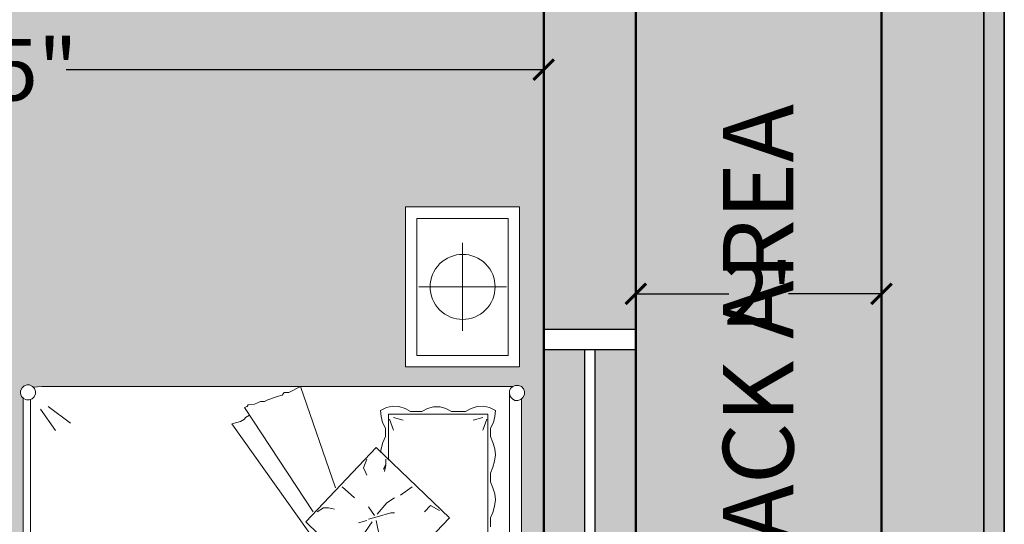
# Model space of a CAD drawing. Units: inches. Extents: x 528 to 2620, y -1066 to 798.
# Tile 15 of 41: x 848 to 944, y 623 to 672. Entities that reach past the tile are written whole.
import ezdxf

# ---------------------------------------------------------------- set-up
doc = ezdxf.new("R2010")
doc.units = ezdxf.units.IN
doc.header["$MEASUREMENT"] = 0
for name, color, linetype, lineweight in [('A-ANNO-DIMS', 2, 'Continuous', 18), ('A-AREA-IDEN', 7, 'Continuous', 18), ('A-FURN', 30, 'Continuous', 18), ('A-GLAZ', 3, 'Continuous', 25), ('A-WALL', 7, 'Continuous', 50), ('A-WALL-PATT', 8, 'Continuous', 13), ('C-PROP', 5, 'Continuous', 35)]:
    doc.layers.add(name, color=color, linetype=linetype, lineweight=lineweight)
doc.styles.get("Standard").update_dxf_attribs({"font": 'arial.ttf'})
doc.dimstyles.get("Standard").update_dxf_attribs({"dimtxt": 6, "dimasz": 2, "dimexe": 0.18, "dimexo": 0.0625, "dimgap": 0.09, "dimtad": 0, "dimtih": 1, "dimtoh": 1, "dimdec": 1, "dimzin": 0, "dimdsep": 46, "dimlunit": 3, "dimtxsty": 'Standard', "dimblk": 'ARCHTICK', "dimcen": 0.09, "dimadec": 0, "dimazin": 0, "dimtfac": 1, "dimtdec": 1, "dimtofl": 0, "dimtmove": 0, "dimatfit": 3, "dimfxl": 1, "dimtolj": 1, "dimtzin": 0, "dimarcsym": 0})

# ---------------------------------------------------------------- blocks, each defined once
blk = doc.blocks.new('d-bed-3')
at = {"color": 0, "linetype": 'ByBlock'}
for p, q in [((0, 0), (0, -0.5)), ((0.7, 0), (0, 0)), ((0.7, -0.5), (0.7, 0)), ((0.7817, -0.0054), (0.7857, 0.0078)), ((0.7817, -0.0054), (0.7857, 0.0078)), ((0.7857, 0.0078), (0.7968, 0.0166)), ((0.7857, 0.0078), (0.7968, 0.0166)), ((0.7968, 0.0166), (0.8078, 0.0211)), ((0.7968, 0.0166), (0.8078, 0.0211)), ((0.8078, 0.0211), (0.8209, 0.0211)), ((0.8078, 0.0211), (0.8209, 0.0211)), ((0.8209, 0.0211), (0.8349, 0.0144)), ((0.8209, 0.0211), (0.8349, 0.0144)), ((0.8349, 0.0144), (0.8409, 0.0078)), ((0.8349, 0.0144), (0.8429, 0.0056)), ((0.8389, 0.0078), (2.7305, 0.0078)), ((0.8409, 0.0078), (2.7305, 0.0078)), ((0.8429, 0.0056), (0.848, -0.0077)), ((0.7817, -0.0187), (0.7817, -0.0054)), ((0.7817, -0.0187), (0.7817, -0.0054)), ((0.7857, -0.0297), (0.7817, -0.0187)), ((0.7857, -0.0297), (0.7817, -0.0187)), ((0.7857, -2.0939), (0.7857, -0.0297)), ((0.7948, -0.0408), (0.7857, -0.0297)), ((0.7857, -0.032), (0.7857, -2.0939)), ((0.8058, -0.0452), (0.7948, -0.0408)), ((0.8319, -0.0408), (0.8188, -0.0452)), ((0.8409, -0.032), (0.8319, -0.0408)), ((0.848, -0.0209), (0.8409, -0.032)), ((0.848, -0.0077), (0.848, -0.0209)), ((0.05, -0.05), (0.05, -0.45)), ((0.65, -0.05), (0.05, -0.05)), ((0.35, -0.0576), (0.35, -0.4424)), ((0.65, -0.45), (0.65, -0.05)), ((0.8188, -0.0452), (0.8058, -0.0452)), ((2.7525, -0.0452), (0.8188, -0.0452)), ((0.8781, -0.1325), (0.8911, -0.1059)), ((0.8911, -0.1059), (0.9182, -0.1082)), ((0.9182, -0.1082), (0.9443, -0.1148)), ((0.9443, -0.1148), (0.9684, -0.128)), ((0.9684, -0.128), (1.0056, -0.128)), ((1.0056, -0.128), (1.0317, -0.117)), ((1.0317, -0.117), (1.0588, -0.1082)), ((1.0588, -0.1082), (1.0849, -0.1059)), ((1.0849, -0.1059), (1.113, -0.1104)), ((1.113, -0.1104), (1.1401, -0.117)), ((1.1401, -0.117), (1.1662, -0.128)), ((1.1662, -0.128), (1.2034, -0.128)), ((1.2034, -0.128), (1.2295, -0.117)), ((1.2295, -0.117), (1.2566, -0.1082)), ((1.2566, -0.1082), (1.2827, -0.1059)), ((1.2827, -0.1059), (1.3108, -0.1104)), ((1.3108, -0.1104), (1.3379, -0.117)), ((1.3379, -0.117), (1.362, -0.128)), ((1.362, -0.128), (1.4012, -0.128)), ((0.8721, -0.159), (0.8781, -0.1325)), ((0.8741, -0.1866), (0.8721, -0.159)), ((0.9072, -0.5753), (0.9072, -0.1391)), ((0.9072, -0.1391), (1.6763, -0.1391)), ((0.9223, -0.1612), (0.9333, -0.2042)), ((0.9293, -0.1435), (0.9775, -0.1612)), ((0.8831, -0.2131), (0.8741, -0.1866)), ((0.8962, -0.2374), (0.8831, -0.2131)), ((0.1576, -0.25), (0.5424, -0.25)), ((0.8962, -0.2992), (0.8962, -0.2374)), ((0.8831, -0.3235), (0.8962, -0.2992)), ((0.8761, -0.3489), (0.8831, -0.3235)), ((1.0538, -0.6294), (1.362, -0.3081)), ((1.362, -0.3081), (1.619, -0.5532)), ((0.8761, -0.3776), (0.8761, -0.3489)), ((0.8831, -0.4041), (0.8761, -0.3776)), ((1.3289, -0.3511), (1.3068, -0.3909)), ((0.8962, -0.4284), (0.8831, -0.4041)), ((0.8962, -0.4781), (0.8962, -0.4284)), ((1.3068, -0.3909), (1.3349, -0.4174)), ((0.05, -0.45), (0.65, -0.45)), ((1.2255, -0.4715), (1.2626, -0.5223)), ((0, -0.5), (0.7, -0.5)), ((0.8741, -0.5289), (0.8831, -0.5024)), ((0.8831, -0.5024), (0.8962, -0.4781)), ((0.9223, -0.5532), (0.9333, -0.5113)), ((0.8721, -0.5576), (0.8741, -0.5289)), ((0.8781, -0.5841), (0.8721, -0.5576)), ((0.9293, -0.5709), (0.9775, -0.5532)), ((1.2957, -0.5819), (1.2737, -0.5488)), ((1.3399, -0.5643), (1.3399, -0.5488)), ((0.8911, -0.6096), (0.8781, -0.5841)), ((1.109, -0.5753), (0.9072, -0.5753)), ((0.9443, -0.6007), (0.9182, -0.6073)), ((0.9684, -0.5886), (0.9443, -0.6007)), ((1.0056, -0.5886), (0.9684, -0.5886)), ((1.0317, -0.5996), (1.0056, -0.5886)), ((1.0588, -0.6073), (1.0317, -0.5996)), ((1.105, -0.5864), (1.1271, -0.5864)), ((1.1271, -0.5864), (1.1482, -0.5974)), ((1.1482, -0.5974), (1.1311, -0.5864)), ((1.1311, -0.5864), (1.1592, -0.593)), ((1.3459, -0.625), (1.2957, -0.5819)), ((1.357, -0.625), (1.3399, -0.5643)), ((0.9182, -0.6073), (0.8911, -0.6096)), ((1.3791, -0.9365), (1.0538, -0.6294)), ((1.0759, -0.6096), (1.0588, -0.6073)), ((1.3138, -0.6626), (1.351, -0.6361)), ((1.368, -0.6626), (1.357, -0.625)), ((1.3731, -0.6294), (1.4453, -0.614)), ((1.3791, -0.6471), (1.4453, -0.6913)), ((1.105, -0.6692), (1.1421, -0.6846)), ((1.1421, -0.6846), (1.1642, -0.6736)), ((1.1642, -0.6736), (1.1753, -0.6692)), ((1.3731, -0.6692), (1.3841, -0.7067)), ((1.2255, -0.7785), (1.2737, -0.7244)), ((1.3791, -0.9365), (1.5357, -0.7763)), ((0.7857, -0.9607), (1.2295, -0.8072)), ((0.9504, -1.2611), (1.5708, -0.8183)), ((1.3178, -0.8382), (1.3239, -0.8117)), ((1.3178, -0.8602), (1.3178, -0.8382)), ((1.3349, -0.8879), (1.3178, -0.8602)), ((0.8781, -1.2059), (1.3349, -0.9055)), ((0.8128, -1.0115), (0.7857, -0.9607)), ((0.8128, -1.0325), (0.8128, -1.0115)), ((0.8239, -1.0414), (0.8128, -1.0325)), ((0.8299, -1.0635), (0.8239, -1.0414)), ((0.8349, -1.0745), (0.8299, -1.0635)), ((0.845, -1.1032), (0.8349, -1.0745)), ((0.852, -1.1187), (0.845, -1.1032)), ((0.852, -1.1363), (0.852, -1.1187)), ((0.863, -1.1617), (0.852, -1.1363)), ((0.867, -1.1905), (0.863, -1.1617)), ((0.8741, -1.1949), (0.867, -1.1905)), ((0.8781, -1.2059), (0.8741, -1.1949)), ((0.9223, -1.2015), (0.9112, -1.1838)), ((0.9293, -1.2059), (0.9223, -1.2015)), ((0.9403, -1.2236), (0.9293, -1.2059)), ((0.9443, -1.2391), (0.9403, -1.2236)), ((0.9504, -1.2611), (0.9443, -1.2391)), ((0.8741, -2.0673), (0.9464, -1.9691)), ((0.8851, -2.1005), (0.9795, -2.0342)), ((0.7888, -2.1317), (0.7857, -2.0939)), ((0.7857, -2.0939), (0.7887, -2.1303)), ((0.7797, -2.148), (0.7857, -2.1347)), ((0.7797, -2.148), (0.7857, -2.1347)), ((0.7797, -2.159), (0.7797, -2.148)), ((0.7797, -2.148), (0.7797, -2.159)), ((0.7857, -2.1347), (0.7948, -2.1259)), ((0.7857, -2.1347), (0.7888, -2.1317)), ((0.7948, -2.1259), (0.8078, -2.1215)), ((0.8078, -2.1215), (0.8188, -2.1215)), ((0.8188, -2.1215), (0.8319, -2.1281)), ((0.8319, -2.1281), (0.8409, -2.1369)), ((0.8409, -2.1369), (0.845, -2.1502)), ((2.7264, -2.1436), (0.845, -2.1436)), ((0.845, -2.1502), (0.845, -2.1612)), ((0.7837, -2.1723), (0.7797, -2.159)), ((0.7837, -2.1723), (0.7797, -2.159)), ((0.7927, -2.1811), (0.7837, -2.1723)), ((0.7927, -2.1811), (0.7837, -2.1723)), ((0.8058, -2.1877), (0.7927, -2.1811)), ((0.8058, -2.1877), (0.7927, -2.1811)), ((0.8168, -2.1877), (0.8058, -2.1877)), ((0.8168, -2.1877), (0.8058, -2.1877)), ((0.8299, -2.1833), (0.8168, -2.1877)), ((0.8299, -2.1833), (0.8168, -2.1877)), ((0.8389, -2.1745), (0.8299, -2.1833)), ((0.8367, -2.1767), (0.8299, -2.1833)), ((2.7327, -2.1767), (0.8367, -2.1767)), ((0.845, -2.1612), (0.8389, -2.1745)), ((0.8389, -2.1767), (2.7305, -2.1767))]:
    blk.add_line(p, q, dxfattribs=at)
blk.add_ellipse((0.35, -0.25), major_axis=(-0.1007, 0.1007), ratio=1, dxfattribs=at)
blk = doc.blocks.new('_ArchTick')
at = {"color": 0, "linetype": 'ByBlock', "const_width": 0.15}
blk.add_lwpolyline([(-0.5, -0.5), (0.5, 0.5)], dxfattribs=at)
blk = doc.blocks.new('*D27')
at = {"layer": 'A-ANNO-DIMS', "color": 0, "lineweight": -2, "transparency": 16777216}
for p, q in [((778.559, 667.76), (778.559, 666.811)), ((899.059, 667.76), (899.059, 666.811)), ((778.559, 666.991), (825.201, 666.991)), ((899.059, 666.991), (852.418, 666.991))]:
    blk.add_line(p, q, dxfattribs=at)
at = {"layer": 'Defpoints', "color": 0, "transparency": 16777216}
for p in [(778.559, 667.823), (899.059, 667.823), (899.059, 666.991)]:
    blk.add_point(p, dxfattribs=at)
at = {"layer": 'A-ANNO-DIMS', "color": 0, "lineweight": -2, "transparency": 16777216, "xscale": 2, "yscale": 2, "zscale": 2, "rotation": 180}
blk.add_blockref('_ArchTick', (778.559, 666.991), dxfattribs=at)
at = {"layer": 'A-ANNO-DIMS', "color": 0, "lineweight": -2, "transparency": 16777216, "xscale": 2, "yscale": 2, "zscale": 2}
blk.add_blockref('_ArchTick', (899.059, 666.991), dxfattribs=at)
at = {"layer": 'A-ANNO-DIMS', "color": 0, "transparency": 16777216, "insert": (838.809, 666.991), "char_height": 6, "attachment_point": 5}
blk.add_mtext('\\A1;10\'-0.5"', dxfattribs=at)
blk = doc.blocks.new('*D39')
at = {"layer": 'A-ANNO-DIMS', "color": 0, "lineweight": -2, "transparency": 16777216}
for p, q in [((908.059, 645.184), (908.059, 645.301)), ((908.059, 645.121), (917.158, 645.121)), ((932.059, 645.121), (922.961, 645.121)), ((932.059, 645.184), (932.059, 645.301))]:
    blk.add_line(p, q, dxfattribs=at)
at = {"layer": 'Defpoints', "color": 0, "transparency": 16777216}
for p in [(908.059, 645.121), (932.059, 645.121), (932.059, 645.121)]:
    blk.add_point(p, dxfattribs=at)
at = {"layer": 'A-ANNO-DIMS', "color": 0, "lineweight": -2, "transparency": 16777216, "xscale": 2, "yscale": 2, "zscale": 2, "rotation": 180}
blk.add_blockref('_ArchTick', (908.059, 645.121), dxfattribs=at)
at = {"layer": 'A-ANNO-DIMS', "color": 0, "lineweight": -2, "transparency": 16777216, "xscale": 2, "yscale": 2, "zscale": 2}
blk.add_blockref('_ArchTick', (932.059, 645.121), dxfattribs=at)
at = {"layer": 'A-ANNO-DIMS', "color": 0, "transparency": 16777216, "insert": (920.059, 645.121), "char_height": 6, "attachment_point": 5}
blk.add_mtext("\\A1;2'", dxfattribs=at)
blk = doc.blocks.new('WIN-1200')
for p, q in [((677.559, 718.922), (725.559, 718.922)), ((677.559, 709.922), (677.559, 718.922)), ((679.559, 709.922), (679.559, 718.922)), ((723.559, 718.922), (723.559, 709.922)), ((725.559, 718.922), (725.559, 709.922)), ((679.559, 714.922), (723.559, 714.922)), ((679.559, 713.922), (723.559, 713.922)), ((725.559, 709.922), (677.559, 709.922))]:
    blk.add_line(p, q)

msp = doc.modelspace()

# ---------------------------------------------------------------- hatches: boundary and pattern name
at = {"layer": 'A-WALL-PATT', "transparency": 33554687}
h = msp.add_hatch(color=256, dxfattribs=at)
h.dxf.hatch_style = 1
h.paths.add_polyline_path([(944.059, 753.922), (584.059, 753.922), (584.059, 208.922), (608.059, 208.922), (608.059, 210.922), (586.059, 210.922), (586.059, 751.922), (942.059, 751.922), (942.059, 210.922), (728.059, 210.922), (728.059, 208.922), (944.059, 208.922)])
h = msp.add_hatch(color=256, dxfattribs=at)
h.dxf.hatch_style = 1
h.paths.add_polyline_path([(942.059, 751.922), (586.059, 751.922), (586.059, 210.922), (608.059, 210.922), (608.059, 220.922), (596.059, 220.922), (596.059, 741.922), (932.059, 741.922), (932.059, 220.922), (770.059, 220.922), (728.059, 220.922), (728.059, 210.922), (942.059, 210.922)])
at = {"layer": 'A-WALL-PATT', "transparency": 33554475}
h = msp.add_hatch(color=256, dxfattribs=at)
h.dxf.hatch_style = 1
h.paths.add_polyline_path([(620.059, 718.922), (908.059, 718.922), (908.059, 268.922), (770.059, 268.922), (770.059, 220.922), (932.059, 220.922), (932.059, 741.922), (596.059, 741.922), (596.059, 391.422), (620.059, 391.422)])
at = {"layer": 'A-WALL-PATT', "transparency": 33554687}
h = msp.add_hatch(color=256, dxfattribs=at)
h.dxf.hatch_style = 1
h.paths.add_polyline_path([(861.059, 273.922), (817.059, 273.922), (817.059, 272.922), (861.059, 272.922)])
h.paths.add_polyline_path([(817.059, 277.922), (815.059, 277.922), (815.059, 268.922), (817.059, 268.922)])
h.paths.add_polyline_path([(908.059, 397.922), (899.059, 397.922), (899.059, 395.922), (908.059, 395.922)])
h.paths.add_polyline_path([(908.059, 443.922), (899.059, 443.922), (899.059, 441.922), (908.059, 441.922)])
h.paths.add_polyline_path([(904.059, 441.922), (903.059, 441.922), (903.059, 397.922), (904.059, 397.922)])
h.paths.add_polyline_path([(625.059, 561.422), (624.059, 561.422), (624.059, 537.422), (625.059, 537.422)])
h.paths.add_polyline_path([(648.747, 334.444), (720.045, 334.444), (720.045, 344.998), (648.747, 344.998)], flags=9)
h.paths.add_polyline_path([(819.733, 323.153), (880.328, 323.153), (880.328, 333.708), (819.733, 333.708)], flags=9)
h.paths.add_polyline_path([(779.898, 680.607), (821.764, 680.607), (821.764, 691.169), (779.898, 691.169)], flags=9)
h.paths.add_polyline_path([(779.876, 692.362), (817.138, 692.362), (817.138, 703.058), (779.876, 703.058)], flags=9)
h.paths.add_polyline_path([(799.994, 453.884), (860.589, 453.884), (860.589, 464.439), (799.994, 464.439)], flags=9)
h.paths.add_polyline_path([(650.866, 539.397), (708.781, 539.397), (708.781, 549.952), (650.866, 549.952)], flags=9)
h.paths.add_polyline_path([(788.504, 612.01), (849.099, 612.01), (849.099, 622.565), (788.504, 622.565)], flags=9)
h.paths.add_polyline_path([(639.539, 648.31), (700.134, 648.31), (700.134, 658.865), (639.539, 658.865)], flags=9)
h.paths.add_polyline_path([(648.913, 346.09), (747.706, 346.09), (747.706, 356.778), (648.913, 356.778)], flags=9)
h.paths.add_polyline_path([(676.857, 450.66), (746.735, 450.66), (746.735, 461.355), (676.857, 461.355)], flags=9)
h.paths.add_polyline_path([(819.711, 334.947), (865.526, 334.947), (865.526, 345.636), (819.711, 345.636)], flags=9)
h.paths.add_polyline_path([(806.298, 467.745), (874.047, 467.745), (874.047, 478.441), (806.298, 478.441)], flags=9)
h.paths.add_polyline_path([(653.235, 552.284), (690.497, 552.284), (690.497, 562.979), (653.235, 562.979)], flags=9)
h.paths.add_polyline_path([(789.903, 623.407), (843.208, 623.407), (843.208, 634.103), (789.903, 634.103)], flags=9)
h.paths.add_polyline_path([(639.773, 662.103), (693.077, 662.103), (693.077, 672.798), (639.773, 672.798)], flags=9)
h.paths.add_polyline_path([(801.587, 242.914), (846.334, 242.914), (846.334, 253.603), (801.587, 253.603)], flags=9)
h.paths.add_polyline_path([(925.362, 593.982), (925.362, 674.057), (914.673, 674.057), (914.673, 593.982)], flags=9)
h.paths.add_polyline_path([(612.559, 593.982), (612.559, 674.057), (601.871, 674.057), (601.871, 593.982)], flags=9)
h.paths.add_polyline_path([(723.31, 726.564), (803.385, 726.564), (803.385, 737.252), (723.31, 737.252)], flags=9)
at = {"layer": 'A-WALL-PATT', "transparency": 33554521}
h = msp.add_hatch(color=256, dxfattribs=at)
h.dxf.hatch_style = 1
h.paths.add_polyline_path([(629.059, 709.922), (677.559, 709.922), (677.559, 718.922), (620.059, 718.922), (620.059, 667.922), (629.059, 667.922)])
h.paths.add_polyline_path([(790.559, 718.922), (725.559, 718.922), (725.559, 709.922), (774.059, 709.922), (774.059, 577.922), (768.481, 577.922), (768.559, 573.422), (774.059, 573.422), (774.059, 567.422), (778.559, 567.422), (778.559, 669.422), (831.059, 669.422), (831.059, 675.922), (826.559, 675.922), (826.559, 673.922), (778.559, 673.922), (778.559, 709.922), (790.559, 709.922)])
h.paths.add_polyline_path([(908.059, 718.922), (879.059, 718.922), (879.059, 709.922), (899.059, 709.922), (899.059, 641.672), (908.059, 641.672)])
h.paths.add_polyline_path([(629.059, 619.922), (620.059, 619.922), (620.059, 561.422), (629.059, 561.422), (629.059, 573.422), (724.059, 573.422), (724.059, 569.422), (728.559, 569.422), (728.559, 577.922), (629.059, 577.922)])
h.paths.add_polyline_path([(779.059, 391.422), (779.059, 400.422), (770.059, 400.422), (764.059, 400.422), (764.059, 397.422), (764.059, 391.422), (770.059, 391.422), (770.059, 268.922), (815.059, 268.922), (815.059, 277.922), (779.059, 277.922), (779.059, 359.767)])
h.paths.add_polyline_path([(908.059, 395.922), (899.059, 395.922), (851.059, 395.922), (851.059, 391.422), (899.059, 391.422), (899.059, 277.922), (863.059, 277.922), (863.059, 268.922), (908.059, 268.922)])
h.paths.add_polyline_path([(908.059, 593.672), (899.059, 593.672), (899.059, 525.422), (778.559, 525.422), (778.559, 527.172), (774.059, 527.172), (774.059, 520.922), (899.059, 520.922), (899.059, 443.922), (908.059, 443.922)])
h.paths.add_polyline_path([(629.059, 520.922), (728.559, 520.922), (728.559, 545.422), (724.059, 545.422), (724.059, 525.422), (629.059, 525.422), (629.059, 537.422), (620.059, 537.422), (620.059, 484.672), (629.059, 484.672)])
h.paths.add_polyline_path([(629.059, 436.672), (620.059, 436.672), (620.059, 391.422), (648.559, 391.422), (648.559, 400.422), (629.059, 400.422)])
h.paths.add_polyline_path([(716.059, 397.422), (716.059, 400.422), (696.559, 400.422), (696.559, 391.422), (716.059, 391.422)])
at = {"layer": 'A-WALL-PATT', "transparency": 33554681}
h = msp.add_hatch(color=256, dxfattribs=at)
h.dxf.hatch_style = 1
h.paths.add_polyline_path([(629.059, 665.922), (625.059, 665.922), (625.059, 621.922), (629.059, 621.922)])
h.paths.add_polyline_path([(624.059, 665.922), (620.059, 665.922), (620.059, 621.922), (624.059, 621.922)])
h.paths.add_polyline_path([(723.559, 713.922), (679.559, 713.922), (679.559, 709.922), (723.559, 709.922)])
h.paths.add_polyline_path([(723.559, 718.922), (679.559, 718.922), (679.559, 714.922), (723.559, 714.922)])
h.paths.add_polyline_path([(814.559, 713.922), (790.559, 713.922), (790.559, 709.922), (814.559, 709.922)])
h.paths.add_polyline_path([(814.559, 718.922), (790.559, 718.922), (790.559, 714.922), (814.559, 714.922)])
h.paths.add_polyline_path([(877.059, 713.922), (833.059, 713.922), (833.059, 709.922), (877.059, 709.922)])
h.paths.add_polyline_path([(877.059, 718.922), (833.059, 718.922), (833.059, 714.922), (877.059, 714.922)])
h.paths.add_polyline_path([(908.059, 639.672), (904.059, 639.672), (904.059, 595.672), (908.059, 595.672)])
h.paths.add_polyline_path([(903.059, 639.672), (899.059, 639.672), (899.059, 595.672), (903.059, 595.672)])
h.paths.add_polyline_path([(908.059, 441.922), (904.059, 441.922), (904.059, 397.922), (908.059, 397.922)])
h.paths.add_polyline_path([(903.059, 441.922), (899.059, 441.922), (899.059, 397.922), (903.059, 397.922)])
h.paths.add_polyline_path([(861.059, 272.922), (817.059, 272.922), (817.059, 268.922), (861.059, 268.922)])
h.paths.add_polyline_path([(861.059, 277.922), (817.059, 277.922), (817.059, 273.922), (861.059, 273.922)])
h.paths.add_polyline_path([(694.559, 395.422), (650.559, 395.422), (650.559, 391.422), (694.559, 391.422)])
h.paths.add_polyline_path([(694.559, 400.422), (650.559, 400.422), (650.559, 396.422), (694.559, 396.422)])
h.paths.add_polyline_path([(629.059, 482.672), (625.059, 482.672), (625.059, 438.672), (629.059, 438.672)])
h.paths.add_polyline_path([(624.059, 482.672), (620.059, 482.672), (620.059, 438.672), (624.059, 438.672)])
h.paths.add_polyline_path([(629.059, 561.422), (625.059, 561.422), (625.059, 537.422), (629.059, 537.422)])
h.paths.add_polyline_path([(624.059, 561.422), (620.059, 561.422), (620.059, 537.422), (624.059, 537.422)])
at = {"layer": 'A-WALL-PATT', "transparency": 33554590}
h = msp.add_hatch(color=256, dxfattribs=at)
h.dxf.hatch_style = 1
h.paths.add_polyline_path([(774.059, 709.922), (629.059, 709.922), (629.059, 577.922), (728.559, 577.922), (728.559, 579.422), (728.559, 619.422), (730.309, 619.422), (730.309, 619.384, -0.401453), (768.559, 579.422), (768.559, 577.922), (774.059, 577.922)])
h.paths.add_polyline_path([(723.896, 686.058), (723.968, 686.064), (723.828, 686.128)], flags=0)
h.paths.add_polyline_path([(722.785, 642.699), (722.893, 642.756), (722.893, 684.992), (722.647, 685.244), (722.647, 685.82), (723.079, 686.262), (723.533, 686.262), (723.968, 686.064), (724.739, 686.128), (770.696, 686.128), (770.78, 686.14), (771.126, 686.266), (771.694, 686.094), (771.94, 685.478), (771.67, 684.904), (771.582, 684.871), (771.582, 642.782), (771.878, 642.514), (771.878, 641.921), (771.511, 641.462), (770.855, 641.462), (770.401, 641.833), (770.401, 641.551), (724.739, 641.551), (723.991, 641.705), (723.443, 641.414), (722.879, 641.585), (722.597, 642.142)], flags=16)
h.paths.add_polyline_path([(723.994, 641.704), (723.994, 641.707), (723.991, 641.705)], flags=0)
h.paths.add_polyline_path([(722.893, 642.732), (722.893, 684.992), (722.647, 685.244), (722.647, 685.82), (723.079, 686.262), (723.287, 686.262), (722.991, 686.172), (722.794, 685.971), (722.647, 685.68), (722.647, 685.434), (722.745, 685.143), (722.942, 684.942), (723.238, 684.807), (723.484, 684.807), (723.779, 684.897), (723.976, 685.098), (724.174, 685.488), (724.124, 685.635), (724.124, 685.249), (723.631, 684.746), (723.631, 642.961), (724.124, 642.514), (724.124, 641.887), (723.656, 641.462), (723.079, 641.462), (722.647, 641.904), (722.647, 642.48)], flags=0)
h.paths.add_polyline_path([(722.647, 642.29), (722.647, 642.044), (722.794, 641.753), (723.079, 641.462), (723.287, 641.462), (722.879, 641.585), (722.597, 642.142)], flags=0)
h.paths.add_polyline_path([(770.745, 686.128), (770.58, 686.128), (770.551, 686.057)], flags=0)
h.paths.add_polyline_path([(743.299, 645.288), (753.227, 659.398), (748.69, 663.75), (753.234, 668.538), (743.299, 682.458), (743.791, 682.592), (744.136, 682.681), (744.53, 682.928), (744.628, 683.084), (745.017, 683.327), (744.53, 684.069), (744.776, 684.158), (744.874, 684.315), (745.514, 684.404), (746.081, 684.651), (746.474, 684.651), (746.819, 684.807), (747.459, 685.031), (747.705, 685.143), (748.198, 685.277), (748.394, 685.523), (748.862, 685.523), (749.994, 686.128), (753.488, 676.03), (757.379, 680.153), (757.791, 679.758), (758.044, 680.645), (758.29, 681.227), (758.29, 682.055), (758.019, 682.592), (757.871, 683.174), (757.822, 683.778), (758.388, 684.069), (758.979, 684.203), (759.619, 684.158), (760.21, 683.957), (760.751, 683.666), (761.859, 683.666), (762.401, 683.957), (762.991, 684.114), (763.631, 684.114), (764.198, 683.957), (764.739, 683.666), (766.118, 683.666), (766.659, 683.957), (767.25, 684.158), (767.865, 684.203), (768.456, 684.069), (769.047, 683.778), (768.998, 683.174), (768.85, 682.592), (768.554, 682.055), (768.554, 681.227), (768.801, 680.645), (769.092, 679.75), (768.948, 678.832), (768.801, 678.228), (768.554, 677.646), (768.554, 676.818), (768.801, 676.237), (769.092, 675.341), (768.948, 674.424), (768.801, 673.82), (768.554, 673.283), (768.554, 672.41), (768.801, 671.873), (768.998, 671.291), (769.047, 670.642), (768.948, 670.016), (768.801, 669.411), (768.554, 668.874), (768.554, 668.002), (768.974, 667.239), (769.047, 666.279), (769.047, 665.563), (768.456, 665.316), (767.865, 665.16), (767.25, 665.16), (766.659, 665.361), (766.118, 665.697), (764.739, 665.697), (763.945, 665.204), (762.991, 665.204), (762.401, 665.361), (761.859, 665.697), (761.005, 665.697), (762.696, 664.086), (760.741, 662.027), (761.859, 662.027), (762.401, 662.318), (763.342, 662.548), (764.247, 662.318), (764.788, 662.027), (766.118, 662.027), (766.659, 662.318), (767.25, 662.519), (767.865, 662.564), (768.505, 662.43), (769.047, 662.116), (769.047, 661.4), (769.047, 660.796), (768.85, 660.214), (768.554, 659.677), (768.554, 658.849), (768.85, 658.267), (768.998, 657.663), (769.069, 656.749), (768.85, 655.851), (768.554, 655.269), (768.554, 654.441), (768.85, 653.859), (769.069, 652.961), (768.998, 652.046), (768.85, 651.442), (768.554, 650.905), (768.554, 650.032), (768.85, 649.495), (768.998, 648.914), (769.047, 648.265), (768.998, 647.638), (768.85, 647.034), (768.554, 646.497), (768.554, 645.624), (768.85, 645.087), (769.047, 644.55), (769.047, 643.901), (768.505, 643.655), (767.865, 643.521), (767.25, 643.521), (766.659, 643.722), (766.118, 644.058), (764.788, 644.058), (764.247, 643.722), (763.342, 643.492), (762.401, 643.722), (761.859, 644.058), (760.801, 644.058), (760.259, 643.722), (759.668, 643.521), (759.028, 643.521), (758.388, 643.655), (757.871, 643.901), (757.871, 644.55), (758.044, 645.087), (758.339, 645.624), (758.339, 646.497), (758.044, 647.034), (757.921, 647.638), (757.866, 648.059), (757.379, 647.593), (753.422, 651.773), (749.994, 641.618), (749.502, 641.708), (749.354, 641.954), (748.542, 642.446), (747.311, 642.939), (746.652, 642.939), (746.327, 643.185), (745.514, 643.565), (744.53, 643.655), (745.011, 644.4), (744.628, 644.639), (744.136, 644.886), (743.791, 645.132)], flags=0)
h.paths.add_polyline_path([(755.656, 654.933), (756.542, 654.687), (757.527, 654.329), (756.641, 654.575)], flags=0)
h.paths.add_polyline_path([(758.339, 649.204), (758.339, 648.712), (758.585, 644.304), (758.585, 648.802)], flags=0)
h.paths.add_polyline_path([(758.339, 649.294), (758.093, 649.697), (758.359, 649.165)], flags=0)
h.paths.add_polyline_path([(755.656, 672.79), (756.493, 673.037), (757.358, 673.351), (757.353, 673.358), (756.641, 673.149)], flags=0)
h.paths.add_polyline_path([(760.264, 639.641), (771.408, 639.641), (771.408, 624.039), (760.264, 624.039)], flags=16)
h.paths.add_polyline_path([(761.378, 638.526), (770.294, 638.526), (770.294, 625.153), (761.378, 625.153)], flags=0)
edge = h.paths.add_edge_path(flags=0)
edge.add_ellipse((765.836, 631.84), major_axis=(-2.245, 2.245), ratio=1, start_angle=-45, end_angle=45, ccw=False)
edge.add_ellipse((765.836, 631.84), major_axis=(-2.245, 2.245), ratio=1, start_angle=-135, end_angle=-45, ccw=False)
edge.add_ellipse((765.836, 631.84), major_axis=(-2.245, 2.245), ratio=1, start_angle=135, end_angle=-135, ccw=False)
edge.add_ellipse((765.836, 631.84), major_axis=(-2.245, 2.245), ratio=1, start_angle=45, end_angle=135, ccw=False)
h.paths.add_polyline_path([(758.585, 683.42), (758.585, 678.922), (758.373, 678.575), (758.339, 678.43), (758.093, 678.049), (758.339, 678.519), (758.339, 679.011)], flags=0)
h.paths.add_polyline_path([(760.264, 688.038), (760.264, 703.64), (771.408, 703.64), (771.408, 688.038)], flags=16)
h.paths.add_polyline_path([(770.401, 685.389), (770.401, 685.846), (770.855, 686.217), (771.511, 686.217), (771.878, 685.758), (771.878, 685.165), (771.582, 684.897), (771.582, 642.782), (771.878, 642.514), (771.878, 641.921), (771.511, 641.462), (770.855, 641.462), (770.401, 641.833), (770.401, 642.29)], flags=0)
h.paths.add_polyline_path([(770.532, 642.678), (771.052, 643.009), (771.67, 642.775), (771.94, 642.201), (771.694, 641.585), (771.126, 641.413), (770.551, 641.622), (770.347, 642.132)], flags=16)
h.paths.add_polyline_path([(761.378, 689.152), (761.378, 702.526), (770.294, 702.526), (770.294, 689.152)], flags=0)
edge = h.paths.add_edge_path(flags=0)
edge.add_ellipse((765.836, 695.839), major_axis=(2.245, 2.245), ratio=1, start_angle=405, end_angle=495, ccw=False)
edge.add_ellipse((765.836, 695.839), major_axis=(2.245, 2.245), ratio=1, start_angle=675, end_angle=765, ccw=False)
edge.add_ellipse((765.836, 695.839), major_axis=(2.245, 2.245), ratio=1, start_angle=585, end_angle=675, ccw=False)
edge.add_ellipse((765.836, 695.839), major_axis=(2.245, 2.245), ratio=1, start_angle=495, end_angle=585, ccw=False)
h.paths.add_polyline_path([(770.696, 684.897), (770.942, 684.74), (771.41, 684.74), (771.73, 685.031), (771.878, 685.344), (771.878, 685.635), (771.694, 686.094), (771.582, 686.128), (771.878, 685.758), (771.878, 685.165), (771.41, 684.74), (770.849, 684.74)], flags=0)
h.paths.add_polyline_path([(899.059, 709.922), (831.059, 709.922), (831.059, 699.922), (829.809, 699.922), (829.809, 675.922), (831.059, 675.922), (831.059, 669.422), (778.559, 669.422), (778.559, 567.172), (780.059, 567.172), (820.059, 567.172), (820.059, 565.422), (820.021, 565.422, -0.401453), (780.059, 527.172), (778.559, 527.172), (778.559, 525.422), (899.059, 525.422)])
h.paths.add_polyline_path([(849.197, 636.014), (849.269, 636.02), (849.129, 636.084)], flags=0)
h.paths.add_polyline_path([(848.193, 634.948), (847.947, 635.2), (847.947, 635.776), (848.379, 636.218), (848.833, 636.218), (849.269, 636.02), (850.039, 636.084), (895.996, 636.084), (896.081, 636.096), (896.426, 636.222), (896.995, 636.05), (897.241, 635.434), (896.97, 634.86), (896.883, 634.827), (896.883, 592.738), (897.178, 592.47), (897.178, 591.877), (896.811, 591.418), (896.155, 591.418), (895.701, 591.789), (895.701, 591.507), (850.039, 591.507), (849.292, 591.661), (848.744, 591.37), (848.18, 591.541), (847.897, 592.098), (848.086, 592.655), (848.193, 592.712)], flags=16)
h.paths.add_polyline_path([(849.294, 591.66), (849.295, 591.663), (849.292, 591.661)], flags=16)
h.paths.add_polyline_path([(848.193, 634.948), (847.947, 635.2), (847.947, 635.776), (848.379, 636.218), (848.587, 636.218), (848.292, 636.128), (848.095, 635.927), (847.947, 635.636), (847.947, 635.39), (848.046, 635.099), (848.243, 634.897), (848.538, 634.763), (848.784, 634.763), (849.079, 634.853), (849.276, 635.054), (849.474, 635.444), (849.424, 635.591), (849.424, 635.205), (848.932, 634.702), (848.932, 592.917), (849.424, 592.47), (849.424, 591.843), (848.956, 591.418), (848.379, 591.418), (847.947, 591.86), (847.947, 592.436), (848.193, 592.688)], flags=0)
h.paths.add_polyline_path([(847.947, 592.246), (847.947, 592), (848.095, 591.709), (848.379, 591.418), (848.587, 591.418), (848.18, 591.541), (847.897, 592.098)], flags=16)
h.paths.add_polyline_path([(896.046, 636.084), (895.88, 636.084), (895.852, 636.013)], flags=0)
h.paths.add_polyline_path([(868.599, 632.414), (869.092, 632.548), (869.436, 632.637), (869.83, 632.884), (869.929, 633.04), (870.318, 633.283), (869.83, 634.025), (870.076, 634.114), (870.175, 634.271), (870.815, 634.36), (871.381, 634.607), (871.775, 634.607), (872.119, 634.763), (872.759, 634.987), (873.006, 635.099), (873.498, 635.233), (873.695, 635.479), (874.163, 635.479), (875.295, 636.084), (878.788, 625.986), (882.679, 630.109), (883.091, 629.714), (883.344, 630.601), (883.59, 631.183), (883.59, 632.011), (883.319, 632.548), (883.172, 633.13), (883.123, 633.734), (883.689, 634.025), (884.279, 634.159), (884.919, 634.114), (885.51, 633.913), (886.052, 633.622), (887.159, 633.622), (887.701, 633.913), (888.292, 634.07), (888.932, 634.07), (889.498, 633.913), (890.039, 633.622), (891.418, 633.622), (891.959, 633.913), (892.55, 634.114), (893.166, 634.159), (893.756, 634.025), (894.347, 633.734), (894.298, 633.13), (894.15, 632.548), (893.855, 632.011), (893.855, 631.183), (894.101, 630.601), (894.393, 629.706), (894.249, 628.788), (894.101, 628.184), (893.855, 627.602), (893.855, 626.774), (894.101, 626.193), (894.393, 625.297), (894.249, 624.38), (894.101, 623.776), (893.855, 623.239), (893.855, 622.366), (894.101, 621.829), (894.298, 621.247), (894.347, 620.598), (894.249, 619.972), (894.101, 619.367), (893.855, 618.83), (893.855, 617.958), (894.274, 617.195), (894.347, 616.235), (894.347, 615.518), (893.756, 615.272), (893.166, 615.116), (892.55, 615.116), (891.959, 615.317), (891.418, 615.653), (890.039, 615.653), (889.245, 615.16), (888.292, 615.16), (887.701, 615.317), (887.159, 615.653), (886.305, 615.653), (887.996, 614.042), (886.041, 611.983), (887.159, 611.983), (887.701, 612.274), (888.642, 612.504), (889.547, 612.274), (890.089, 611.983), (891.418, 611.983), (891.959, 612.274), (892.55, 612.475), (893.166, 612.52), (893.806, 612.386), (894.347, 612.072), (894.347, 611.356), (894.347, 610.752), (894.15, 610.17), (893.855, 609.633), (893.855, 608.805), (894.15, 608.223), (894.298, 607.619), (894.37, 606.705), (894.15, 605.807), (893.855, 605.225), (893.855, 604.397), (894.15, 603.815), (894.37, 602.917), (894.298, 602.002), (894.15, 601.398), (893.855, 600.861), (893.855, 599.988), (894.15, 599.451), (894.298, 598.87), (894.347, 598.221), (894.298, 597.594), (894.15, 596.99), (893.855, 596.453), (893.855, 595.58), (894.15, 595.043), (894.347, 594.506), (894.347, 593.857), (893.806, 593.611), (893.166, 593.477), (892.55, 593.477), (891.959, 593.678), (891.418, 594.014), (890.089, 594.014), (889.547, 593.678), (888.642, 593.448), (887.701, 593.678), (887.159, 594.014), (886.101, 594.014), (885.559, 593.678), (884.969, 593.477), (884.329, 593.477), (883.689, 593.611), (883.172, 593.857), (883.172, 594.506), (883.344, 595.043), (883.639, 595.58), (883.639, 596.453), (883.344, 596.99), (883.221, 597.594), (883.167, 598.015), (882.679, 597.549), (878.722, 601.729), (875.295, 591.574), (874.803, 591.664), (874.655, 591.91), (873.843, 592.402), (872.612, 592.895), (871.952, 592.895), (871.627, 593.141), (870.815, 593.521), (869.83, 593.611), (870.311, 594.356), (869.929, 594.595), (869.436, 594.842), (869.092, 595.088), (868.599, 595.244), (878.528, 609.354), (873.99, 613.706), (878.535, 618.494)], flags=0)
h.paths.add_polyline_path([(880.956, 622.746), (881.793, 622.993), (882.659, 623.307), (882.654, 623.314), (881.941, 623.104)], flags=0)
h.paths.add_polyline_path([(880.956, 604.889), (881.843, 604.643), (882.827, 604.285), (881.941, 604.531)], flags=16)
h.paths.add_polyline_path([(883.393, 628.005), (883.639, 628.475), (883.639, 628.967), (883.886, 633.376), (883.886, 628.878), (883.674, 628.531), (883.639, 628.386)], flags=0)
h.paths.add_polyline_path([(883.639, 599.16), (883.639, 598.668), (883.886, 594.26), (883.886, 598.758)], flags=16)
h.paths.add_polyline_path([(883.639, 599.25), (883.393, 599.653), (883.659, 599.121)], flags=16)
h.paths.add_polyline_path([(885.564, 637.994), (885.564, 653.596), (896.709, 653.596), (896.709, 637.994)], flags=16)
h.paths.add_polyline_path([(885.564, 589.597), (896.709, 589.597), (896.709, 573.995), (885.564, 573.995)], flags=16)
h.paths.add_polyline_path([(886.679, 639.108), (886.679, 652.482), (895.594, 652.482), (895.594, 639.108)], flags=0)
h.paths.add_polyline_path([(886.679, 588.482), (895.594, 588.482), (895.594, 575.109), (886.679, 575.109)], flags=0)
edge = h.paths.add_edge_path(flags=0)
edge.add_ellipse((891.136, 645.795), major_axis=(2.245, 2.245), ratio=1, start_angle=405, end_angle=495, ccw=False)
edge.add_ellipse((891.136, 645.795), major_axis=(2.245, 2.245), ratio=1, start_angle=675, end_angle=765, ccw=False)
edge.add_ellipse((891.136, 645.795), major_axis=(2.245, 2.245), ratio=1, start_angle=585, end_angle=675, ccw=False)
edge.add_ellipse((891.136, 645.795), major_axis=(2.245, 2.245), ratio=1, start_angle=495, end_angle=585, ccw=False)
edge = h.paths.add_edge_path(flags=0)
edge.add_ellipse((891.136, 581.796), major_axis=(-2.245, 2.245), ratio=1, start_angle=-45, end_angle=45, ccw=False)
edge.add_ellipse((891.136, 581.796), major_axis=(-2.245, 2.245), ratio=1, start_angle=-135, end_angle=-45, ccw=False)
edge.add_ellipse((891.136, 581.796), major_axis=(-2.245, 2.245), ratio=1, start_angle=135, end_angle=-135, ccw=False)
edge.add_ellipse((891.136, 581.796), major_axis=(-2.245, 2.245), ratio=1, start_angle=45, end_angle=135, ccw=False)
h.paths.add_polyline_path([(895.701, 635.345), (895.701, 635.802), (896.155, 636.173), (896.811, 636.173), (897.178, 635.714), (897.178, 635.121), (896.883, 634.853), (896.883, 592.738), (897.178, 592.47), (897.178, 591.877), (896.811, 591.418), (896.155, 591.418), (895.701, 591.789), (895.701, 592.246)], flags=0)
h.paths.add_polyline_path([(895.996, 634.853), (896.243, 634.696), (896.71, 634.696), (897.03, 634.987), (897.178, 635.3), (897.178, 635.591), (896.995, 636.05), (896.883, 636.084), (897.178, 635.714), (897.178, 635.121), (896.71, 634.696), (896.15, 634.696)], flags=0)
h.paths.add_polyline_path([(895.832, 592.634), (896.353, 592.965), (896.97, 592.731), (897.241, 592.157), (896.995, 591.541), (896.426, 591.369), (895.852, 591.578), (895.648, 592.088)], flags=16)
h.paths.add_polyline_path([(725.255, 569.422), (724.059, 569.422), (724.059, 573.422), (629.059, 573.422), (629.059, 525.422), (724.059, 525.422), (724.059, 545.422), (725.255, 545.422)])
h.paths.add_polyline_path([(820.021, 565.422), (780.059, 565.422), (780.059, 567.172), (774.059, 567.172), (774.059, 567.422), (774.059, 573.422), (768.559, 573.422), (768.481, 577.922), (768.559, 577.922), (768.559, 579.422, 0.401453), (730.309, 619.384), (730.309, 579.422), (728.559, 579.422), (728.559, 573.422), (728.559, 569.422), (727.255, 569.422), (727.255, 545.422), (728.559, 545.422), (728.559, 520.922), (665.059, 520.922), (665.059, 436.422), (716.059, 436.422), (716.059, 421.422), (717.809, 421.422), (717.809, 421.358, -0.392996), (740.059, 397.422, -0.392996), (762.309, 421.358), (762.309, 421.422), (764.059, 421.422), (764.059, 400.422), (770.059, 400.422), (779.059, 400.422), (779.059, 391.422), (779.059, 359.767), (795.432, 359.767), (795.432, 294.295), (893.669, 294.295), (893.669, 277.922), (899.059, 277.922), (899.059, 391.422), (851.059, 391.422), (851.059, 395.922), (899.059, 395.922), (899.059, 443.922), (899.059, 520.922), (774.059, 520.922), (774.059, 527.172), (778.559, 527.172), (780.059, 527.172, 0.401453)])
h.paths.add_polyline_path([(774.059, 519.657), (842.122, 519.657), (842.122, 505.072), (788.644, 505.072), (788.644, 474.079), (788.644, 470.433, -0.883215), (779.529, 456.663), (774.971, 456.663, -0.414214), (774.059, 457.575)], flags=16)
h.paths.add_polyline_path([(775.883, 517.834), (840.299, 517.834), (840.299, 514.188), (788.644, 514.188), (788.644, 484.41), (779.529, 484.41), (779.529, 474.079), (775.883, 474.079)], flags=0)
h.paths.add_polyline_path([(706.7, 501.564, -0.254069), (706.7, 493.021), (698.31, 492.555), (698.31, 502.031)], flags=16)
h.paths.add_polyline_path([(691.334, 515.692), (691.8, 507.301), (682.325, 507.301), (682.791, 515.692, -0.254069)], flags=16)
h.paths.add_polyline_path([(695.485, 504.685), (695.485, 479.416), (678.64, 479.416), (678.64, 504.685)], flags=16)
h.paths.add_polyline_path([(706.7, 489.602, -0.254069), (706.7, 481.058), (698.31, 480.592), (698.31, 490.068)], flags=16)
h.paths.add_polyline_path([(675.815, 502.031), (675.815, 492.555), (667.425, 493.021, -0.254069), (667.425, 501.564)], flags=16)
h.paths.add_polyline_path([(691.8, 476.8), (691.334, 468.409, -0.254069), (682.791, 468.409), (682.325, 476.8)], flags=16)
h.paths.add_polyline_path([(675.815, 490.068), (675.815, 480.592), (667.425, 481.058, -0.254069), (667.425, 489.602)], flags=16)
h.paths.add_polyline_path([(764.059, 397.422), (762.309, 397.422), (762.309, 421.358, 0.392996), (740.059, 397.422, 0.392996), (717.809, 421.358), (717.809, 397.422), (716.059, 397.422), (716.059, 391.422), (716.059, 385.422), (764.059, 385.422), (764.059, 391.422)], flags=17)
h.paths.add_polyline_path([(716.059, 436.422), (705.859, 436.422), (705.859, 418.422), (716.059, 418.422), (716.059, 421.422)], flags=17)
h.paths.add_polyline_path([(716.059, 418.422), (705.859, 418.422), (705.859, 400.422), (716.059, 400.422)], flags=17)
h.paths.add_polyline_path([(705.859, 418.422), (695.659, 418.422), (695.659, 400.422), (696.559, 400.422), (705.859, 400.422)], flags=17)
h.paths.add_polyline_path([(705.859, 436.422), (695.659, 436.422), (695.659, 418.422), (705.859, 418.422)], flags=17)
h.paths.add_polyline_path([(695.659, 418.422), (685.459, 418.422), (685.459, 400.422), (695.659, 400.422)], flags=17)
h.paths.add_polyline_path([(695.659, 436.422), (685.459, 436.422), (685.459, 418.422), (695.659, 418.422)], flags=17)
h.paths.add_polyline_path([(685.459, 418.422), (675.259, 418.422), (675.259, 400.422), (685.459, 400.422)], flags=17)
h.paths.add_polyline_path([(685.459, 436.422), (675.259, 436.422), (675.259, 418.422), (685.459, 418.422)], flags=17)
h.paths.add_polyline_path([(675.259, 436.422), (665.059, 436.422), (665.059, 418.422), (675.259, 418.422)])
h.paths.add_polyline_path([(675.259, 418.422), (665.059, 418.422), (665.059, 400.422), (675.259, 400.422)])
h.paths.add_polyline_path([(665.059, 418.422), (646.967, 418.422), (646.991, 436.422), (629.059, 436.422), (629.059, 400.422), (665.059, 400.422)])
h.paths.add_polyline_path([(665.059, 436.422), (646.991, 436.422), (646.967, 418.422), (665.059, 418.422)], flags=17)
h.paths.add_polyline_path([(647.005, 446.622), (629.059, 446.622), (629.059, 436.672), (629.059, 436.422), (646.991, 436.422)])
h.paths.add_polyline_path([(665.059, 446.622), (647.005, 446.622), (646.991, 436.422), (665.059, 436.422)])
h.paths.add_polyline_path([(647.019, 456.822), (629.059, 456.822), (629.059, 446.622), (647.005, 446.622)])
h.paths.add_polyline_path([(665.059, 456.822), (647.019, 456.822), (647.005, 446.622), (665.059, 446.622)])
h.paths.add_polyline_path([(647.032, 467.022), (629.059, 467.022), (629.059, 456.822), (647.019, 456.822)])
h.paths.add_polyline_path([(665.059, 467.022), (647.032, 467.022), (647.019, 456.822), (665.059, 456.822)])
h.paths.add_polyline_path([(665.059, 477.222), (647.046, 477.222), (647.032, 467.022), (665.059, 467.022)])
h.paths.add_polyline_path([(647.046, 477.222), (629.059, 477.222), (629.059, 467.022), (647.032, 467.022)])
h.paths.add_polyline_path([(647.059, 487.222), (629.059, 487.222), (629.059, 477.222), (647.046, 477.222), (647.048, 479.019), (645.53, 483.246), (640.877, 480.371)])
h.paths.add_polyline_path([(665.059, 520.922), (629.059, 520.922), (629.059, 487.222), (647.059, 487.222), (665.059, 487.222)])
h.paths.add_polyline_path([(665.059, 487.222), (647.059, 487.222), (653.224, 480.355), (648.578, 483.242), (647.048, 479.019), (647.046, 477.222), (665.059, 477.222)])

# ---------------------------------------------------------------- linework, layer by layer
at = {"layer": 'A-WALL'}
for p, q in [((932.059, 220.922), (932.059, 741.922)), ((908.059, 268.922), (908.059, 718.922)), ((899.059, 525.422), (899.059, 709.922))]:
    msp.add_line(p, q, dxfattribs=at)
at = {"layer": 'C-PROP'}
for points in [[(728.059, 208.922), (944.059, 208.922), (944.059, 753.922), (584.059, 753.922), (584.059, 208.922), (608.059, 208.922)], [(728.059, 210.922), (942.059, 210.922), (942.059, 751.922), (586.059, 751.922), (586.059, 210.922), (608.059, 210.922)]]:
    msp.add_lwpolyline(points, dxfattribs=at)
msp.add_lwpolyline([(596.059, 741.922), (596.059, 220.922), (932.059, 220.922), (932.059, 741.922)], close=True, dxfattribs=at)

# ---------------------------------------------------------------- block references
at = {"layer": 'A-FURN', "xscale": 22.28859121186505, "yscale": 22.28859121186505, "zscale": 22.28859121186505, "rotation": 270}
msp.add_blockref('d-bed-3', (896.709, 653.596), dxfattribs=at)
at = {"layer": 'A-GLAZ', "rotation": 270.000000000001}
msp.add_blockref('WIN-1200', (189.137, 1319.232), dxfattribs=at)

# ---------------------------------------------------------------- texts
at = {"layer": 'A-AREA-IDEN'}
msp.add_text('SET BACK AREA', height=6.89074, rotation=90, dxfattribs=at).set_placement((923.463, 595.763))

# ---------------------------------------------------------------- dimensions: what is measured, and where the dimension line sits
at = {"layer": 'A-ANNO-DIMS'}
for base, p1, p2, picture, middle in [((899.059, 666.991), (778.559, 667.823), (899.059, 667.823), '*D27', (838.809, 666.991)), ((932.059, 645.121), (908.059, 645.121), (932.059, 645.121), '*D39', (920.059, 645.121))]:
    dim = msp.add_linear_dim(base=base, p1=p1, p2=p2, dimstyle='Standard', override={"dimclrd": 0, "dimclre": 0, "dimclrt": 0}, dxfattribs=at)
    dim.commit()
    dim.dimension.update_dxf_attribs({"geometry": picture, "text_midpoint": middle})

doc.saveas('drawing.dxf')
